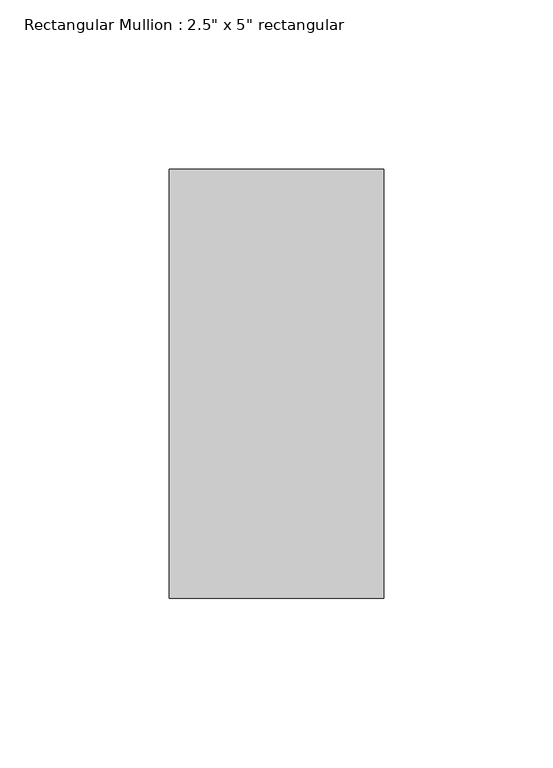
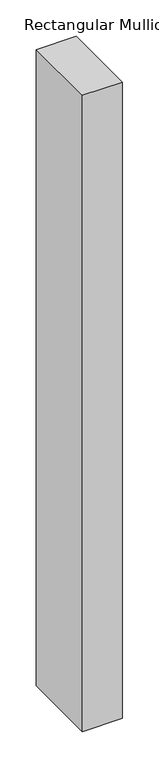
"""IFC4 building model written with IfcOpenShell, lengths in millimetres: member geometry."""

from ifc_helpers import new_model, si_unit, frame, origin, place, context, project, spatial, polyline, outline, extrude, source, transform, mapped, element, save


def member_4194b792(model_context):
    return source(origin(), model_context, "Body", "SweptSolid", [
        extrude(outline(polyline([(31.75, 63.5), (31.75, -63.5), (-31.75, -63.5), (-31.75, 63.5), (31.75, 63.5)])), frame((0.0, 0.0, -1068.9166668), z_axis=(0.0, 0.0, 1.0), x_axis=(1.0, 0.0, 0.0)), (0.0, 0.0, 1.0), 1068.9166668),
    ])


if __name__ == "__main__":
    model = new_model("IFC4")
    model_context = context("Model", 3, world=origin())
    ifc_project = project(units=[si_unit("LENGTHUNIT", "METRE", prefix="MILLI")], contexts=[model_context])
    site = spatial("IfcSite", under=ifc_project)
    building = spatial("IfcBuilding", under=site)
    placement = place(None, origin())
    member_shape = member_4194b792(model_context)
    element("IfcMember", 1, ObjectType="Rectangular Mullion : 2.5\" x 5\" rectangular", at=placement, inside=building, context=model_context, shape_type="MappedRepresentation", body=[
        mapped(member_shape, transform((0.0, 0.0, 0.0), x_axis=(1.0, 0.0, 0.0), y_axis=(0.0, 1.0, 0.0), z_axis=(0.0, 0.0, 1.0))),
    ])
    save(model, "model.ifc")

# Revit data of these elements
# Type "Rectangular Mullion : 2.5\" x 5\" rectangular"
#   built-in parameter 1007304 = 0.416667 (stored number, unit not read)
#   built-in parameter 1007301 = 0.104167 (stored number, unit not read)
#   built-in parameter 1007300 = 0.104167 (stored number, unit not read)
# Element 1 (IfcMember, "Rectangular Mullion : 2.5\" x 5\" rectangular")
#   Materials on its faces: "metal black"
# Materials
#   "metal black": class "Generic", colour RGB 120 120 120, transparency 0, Cost = 0
